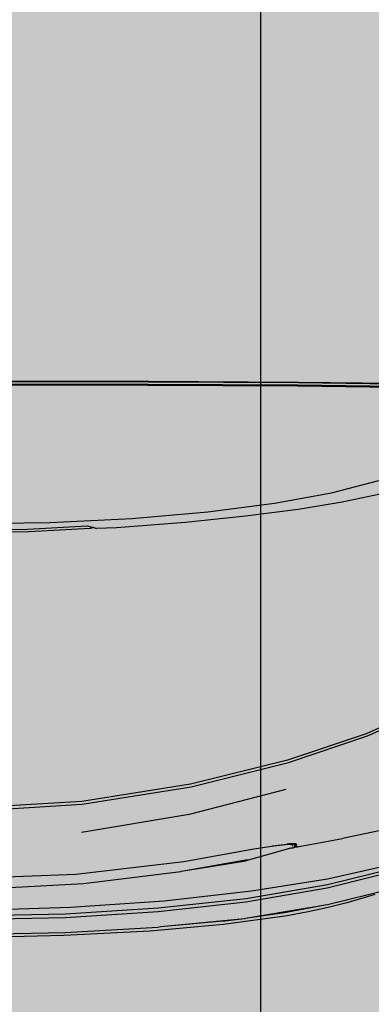
# Model space of a CAD drawing. Units: inches. Extents: x 1884 to 2398, y 474 to 1488.
# Tile 7 of 39: x 2232 to 2247, y 577 to 620. Entities that reach past the tile are written whole.
import ezdxf

# ---------------------------------------------------------------- set-up
doc = ezdxf.new("R2010")
doc.units = ezdxf.units.IN
doc.header["$MEASUREMENT"] = 0
doc.layers.get('0').update_dxf_attribs({"color": 250})
doc.layers.add('A-ANNO-DIMS', color=2, linetype='Continuous', lineweight=18)
doc.layers.add('C-VEHI', color=8, linetype='Continuous', lineweight=18)
doc.layers.add('Edges', color=250, linetype='Continuous')
doc.layers.add('L-PVMT-PATT', color=9, linetype='Continuous', lineweight=13, true_color=0xc7c8ca)
doc.styles.get("Standard").update_dxf_attribs({"font": 'arial.ttf'})
doc.dimstyles.get("Standard").update_dxf_attribs({"dimtxt": 7, "dimasz": 0.18, "dimexe": 0.18, "dimexo": 0.0625, "dimgap": 0.09, "dimtad": 0, "dimtih": 1, "dimtoh": 1, "dimzin": 0, "dimdsep": 46, "dimlunit": 3, "dimtxsty": 'Standard', "dimcen": 0.09, "dimadec": 0, "dimazin": 0, "dimtfac": 1, "dimtofl": 0, "dimtmove": 0, "dimatfit": 3, "dimfxl": 1, "dimtolj": 1, "dimtzin": 0, "dimarcsym": 0})

# ---------------------------------------------------------------- blocks, each defined once
blk = doc.blocks.new('Nissan Qashqai pl')
at = {"layer": 'Edges'}
for p, q in [((11.4138, 12.4223), (11.4422, 12.3594)), ((11.4445, 12.3608), (11.4159, 12.4242)), ((11.056, 12.2851), (11.0572, 12.3942)), ((11.0566, 12.2849), (11.0579, 12.3938)), ((11.0607, 12.3933), (11.0595, 12.2842)), ((11.0618, 12.3933), (11.0606, 12.2841)), ((11.6076, 12.3166), (11.5884, 12.3943)), ((11.5922, 12.3947), (11.6118, 12.3165)), ((11.5467, 12.3822), (11.5571, 12.3331)), ((11.5866, 12.3835), (11.6016, 12.3166)), ((11.6297, 12.3166), (11.6127, 12.3852)), ((11.1776, 12.3211), (11.164, 12.373)), ((11.1791, 12.3746), (11.1877, 12.333)), ((11.6185, 12.3689), (11.6224, 12.3567)), ((11.4422, 12.3594), (11.4712, 12.2729)), ((11.4738, 12.274), (11.4445, 12.3608)), ((11.6224, 12.3567), (11.6277, 12.3379)), ((11.6277, 12.3379), (11.6328, 12.3174)), ((11.1877, 12.333), (11.1958, 12.2844)), ((11.5668, 12.2816), (11.5571, 12.3331)), ((11.1891, 12.2586), (11.1776, 12.3211)), ((11.6016, 12.3166), (11.615, 12.2333)), ((11.6229, 12.2274), (11.6076, 12.3166)), ((11.6118, 12.3165), (11.6272, 12.2272)), ((11.6301, 12.3141), (11.6297, 12.3166)), ((11.6377, 12.2734), (11.6301, 12.3141)), ((11.6332, 12.2951), (11.6301, 12.3141)), ((11.6328, 12.3174), (11.6375, 12.2956)), ((11.6334, 12.2946), (11.6332, 12.2951)), ((11.6443, 12.2288), (11.6334, 12.2946)), ((11.6375, 12.2956), (11.6422, 12.2725)), ((11.0551, 12.1203), (11.056, 12.2851)), ((11.0557, 12.1202), (11.0566, 12.2849)), ((11.0595, 12.2842), (11.0586, 12.1198)), ((11.0606, 12.2841), (11.0597, 12.1196)), ((11.1958, 12.2844), (11.2033, 12.2269)), ((11.5626, 12.2771), (11.5627, 12.2817)), ((11.5627, 12.2817), (11.5634, 12.2829)), ((11.5627, 12.2817), (11.5633, 12.2814)), ((11.5632, 12.2783), (11.5633, 12.2814)), ((11.5633, 12.2814), (11.5634, 12.2829)), ((11.5633, 12.2814), (11.5661, 12.2803)), ((11.5634, 12.2829), (11.5668, 12.2816)), ((11.566, 12.2846), (11.5668, 12.2816)), ((11.5668, 12.2816), (11.5672, 12.2796)), ((11.4712, 12.2729), (11.4976, 12.1662)), ((11.5005, 12.167), (11.4738, 12.274)), ((11.5033, 12.271), (11.5307, 12.165)), ((11.5627, 12.2746), (11.5626, 12.2771)), ((11.5626, 12.2745), (11.5627, 12.2746)), ((11.5628, 12.2721), (11.5627, 12.2746)), ((11.5636, 12.2706), (11.5632, 12.2783)), ((11.5639, 12.2809), (11.5637, 12.2764)), ((11.5637, 12.2763), (11.5637, 12.2764)), ((11.5637, 12.2764), (11.5638, 12.2762)), ((11.5638, 12.2762), (11.5641, 12.2688)), ((11.5643, 12.2808), (11.5639, 12.2809)), ((11.5642, 12.2771), (11.5646, 12.2778)), ((11.566, 12.2801), (11.5643, 12.2808)), ((11.5647, 12.278), (11.5649, 12.2783)), ((11.566, 12.2801), (11.5661, 12.2803)), ((11.5662, 12.28), (11.566, 12.2801)), ((11.5661, 12.2803), (11.5662, 12.28)), ((11.5662, 12.28), (11.5661, 12.2803)), ((11.5669, 12.2797), (11.5661, 12.2803)), ((11.5669, 12.2797), (11.5662, 12.28)), ((11.5662, 12.28), (11.5662, 12.28)), ((11.5667, 12.2813), (11.567, 12.2796)), ((11.567, 12.2796), (11.5669, 12.2797)), ((11.5672, 12.2796), (11.567, 12.2796)), ((11.5678, 12.2766), (11.5672, 12.2796)), ((11.5673, 12.2784), (11.5677, 12.2767)), ((11.5678, 12.2766), (11.5818, 12.227)), ((11.5682, 12.2743), (11.5682, 12.2742)), ((11.5683, 12.2739), (11.5683, 12.2739)), ((11.5683, 12.2738), (11.5683, 12.2737)), ((11.6378, 12.2728), (11.6377, 12.2734)), ((11.6381, 12.2716), (11.6378, 12.2728)), ((11.639, 12.2645), (11.6378, 12.2728)), ((11.639, 12.2645), (11.6381, 12.2716)), ((11.6422, 12.2725), (11.6514, 12.2026)), ((11.565, 12.2577), (11.5636, 12.2706)), ((11.5641, 12.2688), (11.5656, 12.2559)), ((11.6443, 12.2288), (11.639, 12.2645)), ((11.1984, 12.1855), (11.1891, 12.2586)), ((11.5685, 12.2359), (11.565, 12.2577)), ((11.5823, 12.1589), (11.5685, 12.2359)), ((11.593, 12.1566), (11.58, 12.2288)), ((11.615, 12.2333), (11.626, 12.1375)), ((11.6333, 12.131), (11.6229, 12.2274)), ((11.6446, 12.2271), (11.6443, 12.2288)), ((11.2033, 12.2269), (11.21, 12.1607)), ((11.5883, 12.186), (11.5816, 12.2272)), ((11.5883, 12.186), (11.5818, 12.227)), ((11.6272, 12.2272), (11.6377, 12.1308)), ((11.6448, 12.2258), (11.6446, 12.2271)), ((11.6474, 12.2042), (11.6448, 12.2258)), ((11.6539, 12.1338), (11.6448, 12.2258)), ((11.6474, 12.2038), (11.6474, 12.2042)), ((11.6475, 12.2032), (11.6474, 12.2038)), ((11.648, 12.198), (11.6475, 12.2032)), ((11.6539, 12.1338), (11.648, 12.198)), ((11.6514, 12.2026), (11.6589, 12.1222)), ((11.2057, 12.1019), (11.1984, 12.1855)), ((11.593, 12.1566), (11.5883, 12.186)), ((11.4976, 12.1662), (11.5166, 12.0471)), ((11.5196, 12.0475), (11.5005, 12.167)), ((11.5307, 12.165), (11.5504, 12.0466)), ((11.21, 12.1607), (11.2159, 12.085)), ((11.5963, 12.0406), (11.5823, 12.1589)), ((11.5932, 12.1556), (11.593, 12.1566)), ((11.6067, 12.0489), (11.5932, 12.1556)), ((11.626, 12.1375), (11.6329, 12.0344)), ((11.6399, 12.029), (11.6333, 12.131)), ((11.6377, 12.1308), (11.6444, 12.0289)), ((11.6543, 12.1306), (11.6539, 12.1338)), ((11.6604, 12.0287), (11.6543, 12.1306)), ((11.0547, 11.9221), (11.0551, 12.1203)), ((11.0554, 11.9221), (11.0557, 12.1202)), ((11.0586, 12.1198), (11.0583, 11.9221)), ((11.0597, 12.1196), (11.0594, 11.9221)), ((11.6589, 12.1222), (11.6635, 12.0274)), ((11.2101, 12.012), (11.2057, 12.1019)), ((11.2159, 12.085), (11.2166, 12.063)), ((11.2139, 12.0528), (11.2158, 12.0599)), ((11.2158, 12.0602), (11.2166, 12.063)), ((11.2158, 12.0602), (11.2168, 12.056)), ((11.2158, 12.0599), (11.2158, 12.0602)), ((11.2158, 12.0599), (11.2168, 12.056)), ((11.2168, 12.056), (11.2204, 11.989)), ((11.2174, 11.9874), (11.2139, 12.0528)), ((11.5166, 12.0471), (11.5239, 11.9221)), ((11.527, 11.9221), (11.5196, 12.0475)), ((11.6133, 11.9221), (11.6067, 12.0489)), ((11.6005, 11.9335), (11.5963, 12.0406)), ((11.6329, 12.0344), (11.6363, 11.9221)), ((11.6421, 11.9221), (11.6399, 12.029)), ((11.6444, 12.0289), (11.6465, 11.9221)), ((11.6623, 11.9221), (11.6604, 12.0287)), ((11.6635, 12.0274), (11.6663, 11.9221)), ((11.2116, 11.9221), (11.2101, 12.012)), ((11.218, 11.9221), (11.2174, 11.9874)), ((11.2204, 11.989), (11.2211, 11.9221))]:
    blk.add_line(p, q, dxfattribs=at)
blk = doc.blocks.new('car')
blk.add_blockref('Nissan Qashqai pl', (-9.7433, -11.9151))
blk = doc.blocks.new('carr')
blk.add_blockref('car', (0.5124, -0.007))
blk = doc.blocks.new('*D44')
at = {"layer": 'A-ANNO-DIMS', "color": 0, "lineweight": -2, "transparency": 16777216}
for p, q in [((2209.755, 1247.822), (2209.755, 484.005)), ((2230.029, 1247.822), (2230.029, 484.005)), ((2209.935, 484.185), (2229.849, 484.185)), ((2230.029, 484.185), (2230.209, 484.185))]:
    blk.add_line(p, q, dxfattribs=at)
at = {"layer": 'A-ANNO-DIMS', "color": 0, "lineweight": 100, "transparency": 16777216}
for points in [[(2209.935, 484.215), (2209.935, 484.155), (2209.755, 484.185)], [(2229.849, 484.215), (2229.849, 484.155), (2230.029, 484.185)]]:
    blk.add_solid(points, dxfattribs=at)
at = {"layer": 'Defpoints', "color": 0, "lineweight": 100, "transparency": 16777216}
for p in [(2209.755, 1247.885), (2230.029, 1247.885), (2230.029, 484.185)]:
    blk.add_point(p, dxfattribs=at)
at = {"layer": 'A-ANNO-DIMS', "color": 0, "transparency": 16777216, "insert": (2247.429, 484.185), "char_height": 7, "attachment_point": 5}
blk.add_mtext('\\A1;1\'-8 1/2"', dxfattribs=at)
blk = doc.blocks.new('*D45')
at = {"layer": 'A-ANNO-DIMS', "color": 0, "lineweight": -2, "transparency": 16777216}
for p, q in [((2242.617, 1322.822), (2242.617, 484.005)), ((2263.617, 1322.822), (2263.617, 484.005)), ((2242.797, 484.185), (2244.052, 484.185)), ((2263.437, 484.185), (2262.181, 484.185))]:
    blk.add_line(p, q, dxfattribs=at)
at = {"layer": 'A-ANNO-DIMS', "color": 0, "lineweight": 100, "transparency": 16777216}
for points in [[(2242.797, 484.215), (2242.797, 484.155), (2242.617, 484.185)], [(2263.437, 484.215), (2263.437, 484.155), (2263.617, 484.185)]]:
    blk.add_solid(points, dxfattribs=at)
at = {"layer": 'Defpoints', "color": 0, "lineweight": 100, "transparency": 16777216}
for p in [(2242.617, 1322.885), (2263.617, 1322.885), (2263.617, 484.185)]:
    blk.add_point(p, dxfattribs=at)
at = {"layer": 'A-ANNO-DIMS', "color": 0, "transparency": 16777216, "insert": (2253.117, 484.185), "char_height": 7, "attachment_point": 5}
blk.add_mtext('\\A1;1\'-9"', dxfattribs=at)

msp = doc.modelspace()

# ---------------------------------------------------------------- hatches: boundary and pattern name
at = {"layer": 'L-PVMT-PATT'}
h = msp.add_hatch(color=256, dxfattribs=at)
h.dxf.hatch_style = 1
h.paths.add_polyline_path([(2387.529, 769.966), (2351.529, 769.966), (2238.447, 769.966), (2238.447, 762.15), (2238.447, 754.445), (2126.529, 754.445), (2126.529, 676.183), (2134.868, 676.183), (2142.673, 676.183), (2142.673, 646.578), (2134.868, 646.578), (2126.529, 646.578), (2126.529, 640.17), (2387.529, 640.17)])
h.paths.add_polyline_path([(2387.529, 631.385), (2303.086, 631.385), (2303.086, 615.671), (2387.529, 615.671)])
h.paths.add_polyline_path([(2387.529, 640.17), (2126.529, 640.17), (2126.529, 631.385), (2387.529, 631.385)])
h.paths.add_polyline_path([(2393.529, 604.13), (2387.529, 604.13), (2387.529, 615.671), (2303.086, 615.671), (2303.086, 607.943), (2249.649, 607.943), (2126.529, 607.943), (2126.529, 533.885), (2393.529, 533.885)])
h.paths.add_polyline_path([(2257.825, 611.008), (2257.83, 611.337), (2257.915, 616.493), (2258.021, 621.805), (2258.146, 627.274), (2258.252, 631.385), (2126.529, 631.385), (2126.529, 611.008)])
h.paths.add_polyline_path([(2258.892, 611.285), (2258.888, 611.008), (2300.247, 611.008), (2300.247, 631.385), (2259.314, 631.385), (2259.206, 627.173), (2259.081, 621.72), (2258.976, 616.424)])
h = msp.add_hatch(color=256, dxfattribs=at)
h.dxf.hatch_style = 1
h.paths.add_polyline_path([(2216.015, 611.008), (2212.351, 611.008), (2212.342, 608.327), (2212.34, 607.943), (2216.046, 607.943), (2216.044, 608.264)])
h.paths.add_polyline_path([(2212.351, 611.008), (2211.081, 611.008), (2210.074, 609.575), (2209.435, 608.376), (2209.305, 607.943), (2212.34, 607.943), (2212.342, 608.327)])
h.paths.add_polyline_path([(2257.742, 611.008), (2249.649, 611.008), (2217.664, 611.008), (2217.692, 608.284), (2217.694, 607.943), (2249.649, 607.943), (2257.712, 607.943), (2257.713, 608.284)])
h.paths.add_polyline_path([(2266.79, 611.008), (2264.592, 611.008), (2265.355, 609.923), (2266.022, 608.672), (2266.241, 607.943), (2266.364, 607.943), (2266.622, 609.602)])
h.paths.add_polyline_path([(2263.055, 611.008), (2259.39, 611.008), (2259.361, 608.264), (2259.359, 607.943), (2263.065, 607.943), (2263.063, 608.327)])
h.paths.add_polyline_path([(2265.331, 609.575), (2264.325, 611.008), (2263.055, 611.008), (2263.063, 608.327), (2263.065, 607.943), (2266.1, 607.943), (2265.97, 608.376)])
h.paths.add_polyline_path([(2272.885, 609.347), (2272.901, 609.457), (2272.902, 609.679), (2272.895, 611.008), (2271.456, 611.008), (2271.351, 610.147), (2271.277, 610.077), (2270.912, 610.081), (2270.481, 610.11), (2270.455, 610.183), (2270.448, 611.008), (2269.23, 611.008), (2269.228, 610.963), (2269.055, 608.458), (2269.014, 607.943), (2272.869, 607.943), (2272.882, 607.958)])
h.paths.add_polyline_path([(2269.228, 610.963), (2269.23, 611.008), (2267.227, 611.008), (2267.038, 609.547), (2266.77, 607.943), (2269.014, 607.943), (2269.055, 608.458)])
h.paths.add_polyline_path([(2293.178, 611.008), (2272.917, 611.008), (2272.925, 609.643), (2272.924, 609.184), (2272.925, 609.03), (2272.921, 607.943), (2293.123, 607.943), (2293.127, 608.565), (2293.159, 610.362)])
h.paths.add_polyline_path([(2302.932, 613.651), (2302.931, 615.98), (2302.91, 623.22), (2302.851, 630.905), (2302.844, 631.385), (2300.247, 631.385), (2300.247, 612.163), (2300.885, 611.925), (2301.121, 611.86), (2301.743, 612.576)])
h.paths.add_polyline_path([(2302.992, 610.861), (2302.993, 612.796), (2302.965, 612.8), (2301.576, 611.546), (2300.954, 610.83), (2300.899, 610.766), (2300.444, 610.894), (2300.139, 611.008), (2299.369, 611.008), (2299.448, 609.776), (2299.311, 611.008), (2299.207, 611.008), (2299.34, 609.722), (2299.553, 607.943), (2300.825, 607.943), (2300.851, 607.993), (2301.87, 609.442)])
h.paths.add_polyline_path([(2298.512, 611.008), (2296.882, 611.008), (2296.979, 609.034), (2297.054, 607.943), (2298.828, 607.943), (2298.736, 608.659)])
h.paths.add_polyline_path([(2294.51, 608.662), (2294.51, 608.662), (2294.362, 610.672), (2294.359, 611.008), (2293.338, 611.008), (2293.331, 610.606), (2293.329, 610.538), (2293.315, 609.691), (2293.305, 607.943), (2294.597, 607.943)])
h.paths.add_polyline_path([(2302.991, 609.68), (2301.718, 608.051), (2301.642, 607.943), (2302.986, 607.943)], flags=17)

# ---------------------------------------------------------------- block references
at = {"layer": 'C-VEHI', "xscale": 39.37007874015748, "yscale": 39.37007874015748, "zscale": 39.37007874015748, "rotation": 270}
msp.add_blockref('carr', (2229.977, 676.232), dxfattribs=at)

# ---------------------------------------------------------------- dimensions: what is measured, and where the dimension line sits
at = {"layer": 'A-ANNO-DIMS'}
for base, p1, p2, picture, middle in [((2263.617, 484.185), (2242.617, 1322.885), (2263.617, 1322.885), '*D45', (2253.117, 484.185)), ((2230.029, 484.185), (2209.755, 1247.885), (2230.029, 1247.885), '*D44', (2247.429, 484.185))]:
    dim = msp.add_linear_dim(base=base, p1=p1, p2=p2, dimstyle='Standard', override={"dimdec": 1, "dimlfac": 1, "dimrnd": 0, "dimzin": 1, "dimdsep": 46, "dimlunit": 4, "dimfrac": 2}, dxfattribs=at)
    dim.commit()
    dim.dimension.update_dxf_attribs({"geometry": picture, "text_midpoint": middle})

doc.saveas('drawing.dxf')
